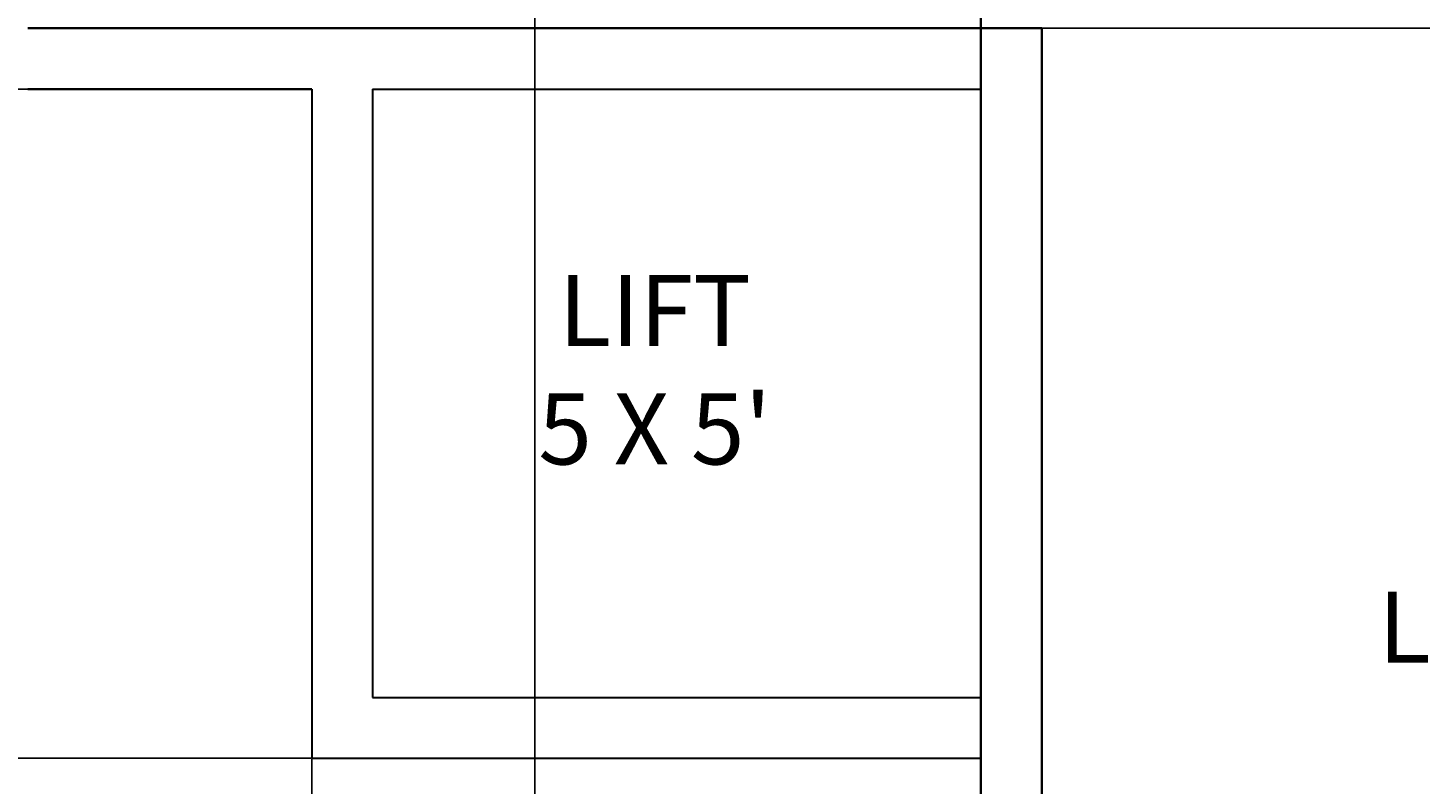
# Model space of a CAD drawing. Units: feet. Extents: x 105 to 1094, y -88 to 588.
# Tile 37 of 59: x 553 to 690, y 138 to 212. Entities that reach past the tile are written whole.
import ezdxf

# ---------------------------------------------------------------- set-up
doc = ezdxf.new("R2010")
doc.units = ezdxf.units.FT
doc.header["$MEASUREMENT"] = 0
for name, color, linetype, lineweight in [('A-ANNO-DIMS', 2, 'Continuous', 18), ('A-AREA-IDEN', 7, 'Continuous', 18), ('A-CONV', 7, 'Continuous', 30), ('A-WALL', 7, 'Continuous', 35)]:
    doc.layers.add(name, color=color, linetype=linetype, lineweight=lineweight)
doc.styles.get("Standard").update_dxf_attribs({"font": 'arial.ttf'})
doc.dimstyles.get("Standard").update_dxf_attribs({"dimtxt": 0.18, "dimasz": 0.18, "dimexe": 0.18, "dimexo": 0.0625, "dimgap": 0.09, "dimtad": 0, "dimtih": 1, "dimtoh": 1, "dimdec": 4, "dimzin": 0, "dimdsep": 46, "dimtxsty": 'Standard', "dimcen": 0.09, "dimadec": 0, "dimazin": 0, "dimtfac": 1, "dimtdec": 4, "dimtofl": 0, "dimtmove": 0, "dimatfit": 3, "dimfxl": 1, "dimtolj": 1, "dimtzin": 0, "dimarcsym": 0})

# ---------------------------------------------------------------- blocks, each defined once
blk = doc.blocks.new('*D20')
at = {"layer": 'A-ANNO-DIMS', "color": 0, "lineweight": -2, "transparency": 16777216}
for p, q in [((150.69, 276.02), (150.69, -88.15)), ((1048.69, 276.02), (1048.69, -88.15)), ((150.87, -87.97), (599.4, -87.97)), ((1048.51, -87.97), (599.98, -87.97))]:
    blk.add_line(p, q, dxfattribs=at)
at = {"layer": 'A-ANNO-DIMS', "color": 0, "transparency": 16777216}
for points in [[(150.87, -87.94), (150.87, -88), (150.69, -87.97)], [(1048.51, -87.94), (1048.51, -88), (1048.69, -87.97)]]:
    blk.add_solid(points, dxfattribs=at)
at = {"layer": 'Defpoints', "color": 0, "transparency": 16777216}
for p in [(150.69, 276.08), (1048.69, 276.08), (1048.69, -87.97)]:
    blk.add_point(p, dxfattribs=at)
at = {"layer": 'A-ANNO-DIMS', "color": 0, "transparency": 16777216, "insert": (599.69, -87.97), "char_height": 0.18, "attachment_point": 5}
blk.add_mtext('\\A1;898', dxfattribs=at)
blk = doc.blocks.new('*D21')
at = {"layer": 'A-ANNO-DIMS', "color": 0, "lineweight": -2, "transparency": 16777216}
for p, q in [((849.63, 543.08), (105.46, 543.08)), ((105.64, 542.9), (105.64, 250.26)), ((105.64, -42.74), (105.64, 249.9)), ((849.63, -42.92), (105.46, -42.92))]:
    blk.add_line(p, q, dxfattribs=at)
at = {"layer": 'A-ANNO-DIMS', "color": 0, "transparency": 16777216}
for points in [[(105.61, 542.9), (105.67, 542.9), (105.64, 543.08)], [(105.61, -42.74), (105.67, -42.74), (105.64, -42.92)]]:
    blk.add_solid(points, dxfattribs=at)
at = {"layer": 'Defpoints', "color": 0, "transparency": 16777216}
for p in [(105.64, 543.08), (849.69, 543.08), (849.69, -42.92)]:
    blk.add_point(p, dxfattribs=at)
at = {"layer": 'A-ANNO-DIMS', "color": 0, "transparency": 16777216, "insert": (105.64, 250.08), "char_height": 0.18, "attachment_point": 5}
blk.add_mtext('\\A1;586', dxfattribs=at)
blk = doc.blocks.new('*D34')
at = {"layer": 'A-ANNO-DIMS', "color": 0, "lineweight": -2, "transparency": 16777216}
for p, q in [((552.75, 295.08), (1093.92, 295.08)), ((1093.74, 294.9), (1093.74, 253.76)), ((1093.74, 212.26), (1093.74, 253.4)), ((552.75, 212.08), (1093.92, 212.08))]:
    blk.add_line(p, q, dxfattribs=at)
at = {"layer": 'A-ANNO-DIMS', "color": 0, "transparency": 16777216}
for points in [[(1093.71, 294.9), (1093.77, 294.9), (1093.74, 295.08)], [(1093.71, 212.26), (1093.77, 212.26), (1093.74, 212.08)]]:
    blk.add_solid(points, dxfattribs=at)
at = {"layer": 'Defpoints', "color": 0, "transparency": 16777216}
for p in [(552.69, 295.08), (552.69, 212.08), (1093.74, 212.08)]:
    blk.add_point(p, dxfattribs=at)
at = {"layer": 'A-ANNO-DIMS', "color": 0, "transparency": 16777216, "insert": (1093.74, 253.58), "char_height": 0.18, "attachment_point": 5}
blk.add_mtext('\\A1;83', dxfattribs=at)
blk = doc.blocks.new('*D35')
at = {"layer": 'A-ANNO-DIMS', "color": 0, "lineweight": -2, "transparency": 16777216}
for p, q in [((580.69, 140.02), (580.69, -88.15)), ((646.69, 140.02), (646.69, -88.15)), ((580.87, -87.97), (613.47, -87.97)), ((646.51, -87.97), (613.91, -87.97))]:
    blk.add_line(p, q, dxfattribs=at)
at = {"layer": 'A-ANNO-DIMS', "color": 0, "transparency": 16777216}
for points in [[(580.87, -87.94), (580.87, -88), (580.69, -87.97)], [(646.51, -87.94), (646.51, -88), (646.69, -87.97)]]:
    blk.add_solid(points, dxfattribs=at)
at = {"layer": 'Defpoints', "color": 0, "transparency": 16777216}
for p in [(580.69, 140.08), (646.69, 140.08), (646.69, -87.97)]:
    blk.add_point(p, dxfattribs=at)
at = {"layer": 'A-ANNO-DIMS', "color": 0, "transparency": 16777216, "insert": (613.69, -87.97), "char_height": 0.18, "attachment_point": 5}
blk.add_mtext('\\A1;66', dxfattribs=at)
blk = doc.blocks.new('*D46')
at = {"layer": 'A-ANNO-DIMS', "color": 0, "lineweight": -2, "transparency": 16777216}
for p, q in [((580.63, 206.08), (105.46, 206.08)), ((105.64, 205.9), (105.64, 173.26)), ((105.64, 140.26), (105.64, 172.9)), ((580.63, 140.08), (105.46, 140.08))]:
    blk.add_line(p, q, dxfattribs=at)
at = {"layer": 'A-ANNO-DIMS', "color": 0, "transparency": 16777216}
for points in [[(105.61, 205.9), (105.67, 205.9), (105.64, 206.08)], [(105.61, 140.26), (105.67, 140.26), (105.64, 140.08)]]:
    blk.add_solid(points, dxfattribs=at)
at = {"layer": 'Defpoints', "color": 0, "transparency": 16777216}
for p in [(580.69, 206.08), (105.64, 140.08), (580.69, 140.08)]:
    blk.add_point(p, dxfattribs=at)
at = {"layer": 'A-ANNO-DIMS', "color": 0, "transparency": 16777216, "insert": (105.64, 173.08), "char_height": 0.18, "attachment_point": 5}
blk.add_mtext('\\A1;66', dxfattribs=at)
blk = doc.blocks.new('*D49')
at = {"layer": 'A-ANNO-DIMS', "color": 0, "lineweight": -2, "transparency": 16777216}
for p, q in [((602.69, 295.02), (602.69, -88.15)), ((646.69, 295.02), (646.69, -88.15)), ((602.87, -87.97), (624.47, -87.97)), ((646.51, -87.97), (624.91, -87.97))]:
    blk.add_line(p, q, dxfattribs=at)
at = {"layer": 'A-ANNO-DIMS', "color": 0, "transparency": 16777216}
for points in [[(602.87, -87.94), (602.87, -88), (602.69, -87.97)], [(646.51, -87.94), (646.51, -88), (646.69, -87.97)]]:
    blk.add_solid(points, dxfattribs=at)
at = {"layer": 'Defpoints', "color": 0, "transparency": 16777216}
for p in [(602.69, 295.08), (646.69, 295.08), (646.69, -87.97)]:
    blk.add_point(p, dxfattribs=at)
at = {"layer": 'A-ANNO-DIMS', "color": 0, "transparency": 16777216, "insert": (624.69, -87.97), "char_height": 0.18, "attachment_point": 5}
blk.add_mtext('\\A1;44', dxfattribs=at)

msp = doc.modelspace()

# ---------------------------------------------------------------- linework, layer by layer
at = {"layer": 'A-CONV'}
for p, q in [((580.6883, 206.0812), (580.6883, 140.0812)), ((586.6883, 206.0812), (586.6883, 146.0812)), ((586.6883, 206.0812), (646.6883, 206.0812)), ((586.6883, 146.0812), (646.6883, 146.0812)), ((580.6883, 140.0812), (646.6883, 140.0812))]:
    msp.add_line(p, q, dxfattribs=at)
at = {"layer": 'A-WALL'}
for p, q in [((646.6883, 248.0812), (646.6883, 140.0812)), ((552.6883, 212.0812), (646.6883, 212.0812)), ((646.6883, 212.0812), (652.6883, 212.0812)), ((646.6883, 59.0812), (646.6883, 212.0812)), ((652.6883, 65.0812), (652.6883, 212.0812)), ((552.6883, 206.0812), (580.6883, 206.0812))]:
    msp.add_line(p, q, dxfattribs=at)

# ---------------------------------------------------------------- texts
at = {"layer": 'A-AREA-IDEN', "char_height": 7}
for s, insert, attachment_point in [("\\pxqc;LIFT\\P5 X 5'", (565.367, 187.728), 1), ('\\pxqc;Living Room \\P10\' x 11\'9"', (664.3247, 137.8526), 7)]:
    msp.add_mtext_dynamic_manual_height_columns(s, width=98.34246, gutter_width=1, heights=[0], dxfattribs=dict(at, insert=insert, attachment_point=attachment_point))

# ---------------------------------------------------------------- dimensions: what is measured, and where the dimension line sits
at = {"layer": 'A-ANNO-DIMS'}
for base, p1, p2, picture, middle in [((105.6383, 543.0812), (849.6883, -42.9188), (849.6883, 543.0812), '*D21', (105.6383, 250.0812)), ((1093.7383, 212.0812), (552.6883, 295.0812), (552.6883, 212.0812), '*D34', (1093.7383, 253.5812)), ((105.6383, 140.0812), (580.6883, 206.0812), (580.6883, 140.0812), '*D46', (105.6383, 173.0812))]:
    dim = msp.add_linear_dim(base=base, p1=p1, p2=p2, angle=90, dimstyle='Standard', override={"dimdec": 0, "dimlfac": 1, "dimrnd": 0, "dimzin": 0, "dimdsep": 46, "dimlunit": 2}, dxfattribs=at)
    dim.commit()
    dim.dimension.update_dxf_attribs({"geometry": picture, "text_midpoint": middle})
for base, p1, p2, picture, middle in [((646.6883, -87.9688), (602.6883, 295.0812), (646.6883, 295.0812), '*D49', (624.6883, -87.9688)), ((1048.6883, -87.9688), (150.6883, 276.0812), (1048.6883, 276.0812), '*D20', (599.6883, -87.9688)), ((646.6883, -87.9688), (580.6883, 140.0812), (646.6883, 140.0812), '*D35', (613.6883, -87.9688))]:
    dim = msp.add_linear_dim(base=base, p1=p1, p2=p2, dimstyle='Standard', override={"dimdec": 0, "dimlfac": 1, "dimrnd": 0, "dimzin": 0, "dimdsep": 46, "dimlunit": 2}, dxfattribs=at)
    dim.commit()
    dim.dimension.update_dxf_attribs({"geometry": picture, "text_midpoint": middle})

doc.saveas('drawing.dxf')
